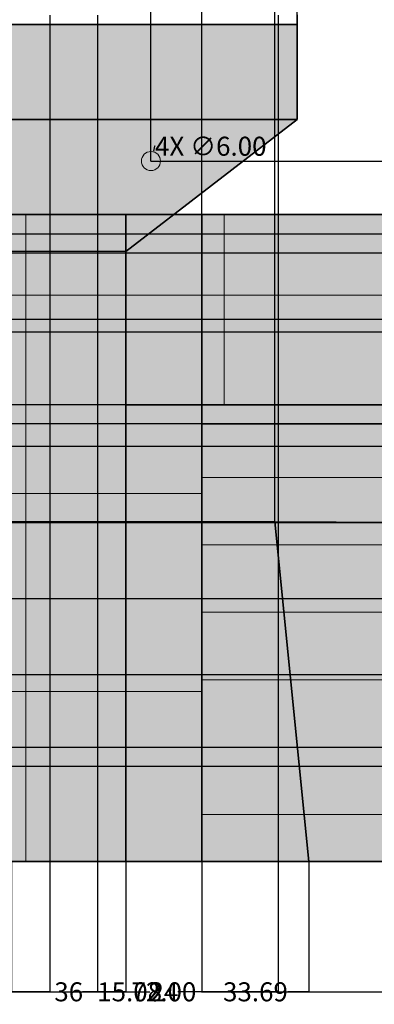
# Model space of a CAD drawing. Units: inches. Extents: x 148 to 1080, y 89 to 707.
# Tile 8 of 12: x 686 to 797, y 89 to 399. Entities that reach past the tile are written whole.
import ezdxf

# ---------------------------------------------------------------- set-up
doc = ezdxf.new("R2010")
doc.units = ezdxf.units.IN
doc.header["$MEASUREMENT"] = 0
for name, color, linetype, lineweight in [('A-ANNO-DIMS', 2, 'Continuous', 18), ('A-ELEV', 7, 'Continuous', 35), ('A-ELEV-PATT', 8, 'Continuous', 13), ('E-LITE', 3, 'Continuous', 18)]:
    doc.layers.add(name, color=color, linetype=linetype, lineweight=lineweight)
doc.styles.get("Standard").update_dxf_attribs({"font": 'arial.ttf'})
doc.dimstyles.get("Standard").update_dxf_attribs({"dimtxt": 6, "dimasz": 0.18, "dimexe": 0.18, "dimexo": 0.0625, "dimgap": 0.09, "dimtad": 0, "dimtih": 1, "dimtoh": 1, "dimdec": 0, "dimzin": 0, "dimdsep": 46, "dimlunit": 3, "dimtxsty": 'Standard', "dimcen": 0.09, "dimadec": 0, "dimazin": 0, "dimtfac": 1, "dimtdec": 0, "dimtofl": 0, "dimtmove": 0, "dimatfit": 3, "dimfxl": 1, "dimtolj": 1, "dimtzin": 0, "dimarcsym": 0})

# ---------------------------------------------------------------- blocks, each defined once
blk = doc.blocks.new('*D1')
at = {"layer": 'A-ANNO-DIMS', "color": 0, "lineweight": -2, "transparency": 16777216}
for p, q in [((215.02, 662.01), (215.02, 703.28)), ((215.2, 703.1), (604.32, 703.1)), ((1006.77, 703.1), (617.65, 703.1)), ((1006.95, 338.01), (1006.95, 703.28))]:
    blk.add_line(p, q, dxfattribs=at)
at = {"layer": 'A-ANNO-DIMS', "color": 0, "transparency": 16777216}
for points in [[(215.2, 703.13), (215.2, 703.07), (215.02, 703.1)], [(1006.77, 703.13), (1006.77, 703.07), (1006.95, 703.1)]]:
    blk.add_solid(points, dxfattribs=at)
at = {"layer": 'Defpoints', "color": 0, "transparency": 16777216}
for p in [(1006.95, 703.1), (215.02, 661.95), (1006.95, 337.95)]:
    blk.add_point(p, dxfattribs=at)
at = {"layer": 'A-ANNO-DIMS', "color": 0, "transparency": 16777216, "insert": (610.98, 703.1), "char_height": 6, "attachment_point": 5}
blk.add_mtext('\\A1;792', dxfattribs=at)
blk = doc.blocks.new('*D4')
at = {"layer": 'A-ANNO-DIMS', "color": 0, "lineweight": -2, "transparency": 16777216}
for p, q in [((683.02, 133.88), (683.02, 92.62)), ((719.02, 133.88), (719.02, 92.62)), ((683.2, 92.8), (696.64, 92.8)), ((718.84, 92.8), (705.4, 92.8))]:
    blk.add_line(p, q, dxfattribs=at)
at = {"layer": 'A-ANNO-DIMS', "color": 0, "transparency": 16777216}
for points in [[(683.2, 92.83), (683.2, 92.77), (683.02, 92.8)], [(718.84, 92.83), (718.84, 92.77), (719.02, 92.8)]]:
    blk.add_solid(points, dxfattribs=at)
at = {"layer": 'Defpoints', "color": 0, "transparency": 16777216}
for p in [(683.02, 133.95), (719.02, 133.95), (719.02, 92.8)]:
    blk.add_point(p, dxfattribs=at)
at = {"layer": 'A-ANNO-DIMS', "color": 0, "transparency": 16777216, "insert": (701.02, 92.8), "char_height": 6, "attachment_point": 5}
blk.add_mtext('\\A1;36', dxfattribs=at)
blk = doc.blocks.new('*D5')
at = {"layer": 'A-ANNO-DIMS', "color": 0, "lineweight": -2, "transparency": 16777216}
for p, q in [((719.02, 133.88), (719.02, 92.62)), ((743.02, 133.88), (743.02, 92.62)), ((719.2, 92.8), (726.59, 92.8)), ((742.84, 92.8), (735.45, 92.8))]:
    blk.add_line(p, q, dxfattribs=at)
at = {"layer": 'A-ANNO-DIMS', "color": 0, "transparency": 16777216}
for points in [[(719.2, 92.83), (719.2, 92.77), (719.02, 92.8)], [(742.84, 92.83), (742.84, 92.77), (743.02, 92.8)]]:
    blk.add_solid(points, dxfattribs=at)
at = {"layer": 'Defpoints', "color": 0, "transparency": 16777216}
for p in [(719.02, 133.95), (743.02, 133.95), (743.02, 92.8)]:
    blk.add_point(p, dxfattribs=at)
at = {"layer": 'A-ANNO-DIMS', "color": 0, "transparency": 16777216, "insert": (731.02, 92.8), "char_height": 6, "attachment_point": 5}
blk.add_mtext('\\A1;24', dxfattribs=at)
blk = doc.blocks.new('*D6')
at = {"layer": 'A-ANNO-DIMS', "color": 0, "lineweight": -2, "transparency": 16777216}
for p, q in [((743.02, 133.88), (743.02, 92.62)), ((946.95, 133.88), (946.95, 92.62)), ((743.2, 92.8), (832.39, 92.8)), ((946.77, 92.8), (857.58, 92.8))]:
    blk.add_line(p, q, dxfattribs=at)
at = {"layer": 'A-ANNO-DIMS', "color": 0, "transparency": 16777216}
for points in [[(743.2, 92.83), (743.2, 92.77), (743.02, 92.8)], [(946.77, 92.83), (946.77, 92.77), (946.95, 92.8)]]:
    blk.add_solid(points, dxfattribs=at)
at = {"layer": 'Defpoints', "color": 0, "transparency": 16777216}
for p in [(743.02, 133.95), (946.95, 133.95), (946.95, 92.8)]:
    blk.add_point(p, dxfattribs=at)
at = {"layer": 'A-ANNO-DIMS', "color": 0, "transparency": 16777216, "insert": (844.98, 92.8), "char_height": 6, "attachment_point": 5}
blk.add_mtext('\\A1;203.93', dxfattribs=at)
blk = doc.blocks.new('*D17')
at = {"layer": 'A-ANNO-DIMS', "color": 0, "lineweight": -2, "transparency": 16777216}
for p, q in [((743.02, 338.01), (743.02, 703.28)), ((743.2, 703.1), (753.64, 703.1)), ((772.84, 703.1), (762.39, 703.1)), ((773.02, 368.01), (773.02, 703.28))]:
    blk.add_line(p, q, dxfattribs=at)
at = {"layer": 'A-ANNO-DIMS', "color": 0, "transparency": 16777216}
for points in [[(743.2, 703.13), (743.2, 703.07), (743.02, 703.1)], [(772.84, 703.13), (772.84, 703.07), (773.02, 703.1)]]:
    blk.add_solid(points, dxfattribs=at)
at = {"layer": 'Defpoints', "color": 0, "transparency": 16777216}
for p in [(773.02, 703.1), (773.02, 367.95), (743.02, 337.95)]:
    blk.add_point(p, dxfattribs=at)
at = {"layer": 'A-ANNO-DIMS', "color": 0, "transparency": 16777216, "insert": (758.02, 703.1), "char_height": 6, "attachment_point": 5}
blk.add_mtext('\\A1;30', dxfattribs=at)
blk = doc.blocks.new('*D18')
at = {"layer": 'A-ANNO-DIMS', "color": 0, "lineweight": -2, "transparency": 16777216}
for p, q in [((635.08, 661.95), (1064.5, 661.95)), ((1064.32, 661.77), (1064.32, 401.1)), ((1064.32, 134.13), (1064.32, 394.79)), ((1007.01, 133.95), (1064.5, 133.95))]:
    blk.add_line(p, q, dxfattribs=at)
at = {"layer": 'A-ANNO-DIMS', "color": 0, "transparency": 16777216}
for points in [[(1064.29, 661.77), (1064.35, 661.77), (1064.32, 661.95)], [(1064.29, 134.13), (1064.35, 134.13), (1064.32, 133.95)]]:
    blk.add_solid(points, dxfattribs=at)
at = {"layer": 'Defpoints', "color": 0, "transparency": 16777216}
for p in [(635.02, 661.95), (1064.32, 661.95), (1006.95, 133.95)]:
    blk.add_point(p, dxfattribs=at)
at = {"layer": 'A-ANNO-DIMS', "color": 0, "transparency": 16777216, "insert": (1064.32, 397.95), "char_height": 6, "attachment_point": 5}
blk.add_mtext('\\A1;528', dxfattribs=at)
blk = doc.blocks.new('*D35')
at = {"layer": 'A-ANNO-DIMS', "color": 0, "lineweight": -2, "transparency": 16777216}
for p, q in [((743.02, 272.01), (743.02, 703.28)), ((743.2, 703.1), (765.77, 703.1)), ((765.95, 241.16), (765.95, 703.28)), ((765.95, 703.1), (766.13, 703.1))]:
    blk.add_line(p, q, dxfattribs=at)
at = {"layer": 'A-ANNO-DIMS', "color": 0, "transparency": 16777216}
for points in [[(743.2, 703.13), (743.2, 703.07), (743.02, 703.1)], [(765.77, 703.13), (765.77, 703.07), (765.95, 703.1)]]:
    blk.add_solid(points, dxfattribs=at)
at = {"layer": 'Defpoints', "color": 0, "transparency": 16777216}
for p in [(765.95, 703.1), (743.02, 271.95), (765.95, 241.1)]:
    blk.add_point(p, dxfattribs=at)
at = {"layer": 'A-ANNO-DIMS', "color": 0, "transparency": 16777216, "insert": (778.73, 703.1), "char_height": 6, "attachment_point": 5}
blk.add_mtext('\\A1;22.928', dxfattribs=at)
blk = doc.blocks.new('*D36')
at = {"layer": 'A-ANNO-DIMS', "color": 0, "lineweight": -2, "transparency": 16777216}
for p, q in [((765.95, 241.16), (765.95, 703.28)), ((766.13, 703.1), (844.01, 703.1)), ((934.77, 703.1), (856.89, 703.1)), ((934.95, 272.01), (934.95, 703.28))]:
    blk.add_line(p, q, dxfattribs=at)
at = {"layer": 'A-ANNO-DIMS', "color": 0, "transparency": 16777216}
for points in [[(766.13, 703.13), (766.13, 703.07), (765.95, 703.1)], [(934.77, 703.13), (934.77, 703.07), (934.95, 703.1)]]:
    blk.add_solid(points, dxfattribs=at)
at = {"layer": 'Defpoints', "color": 0, "transparency": 16777216}
for p in [(934.95, 703.1), (934.95, 271.95), (765.95, 241.1)]:
    blk.add_point(p, dxfattribs=at)
at = {"layer": 'A-ANNO-DIMS', "color": 0, "transparency": 16777216, "insert": (850.45, 703.1), "char_height": 6, "attachment_point": 5}
blk.add_mtext('\\A1;169', dxfattribs=at)
blk = doc.blocks.new('*D37')
at = {"layer": 'A-ANNO-DIMS', "color": 0, "lineweight": -2, "transparency": 16777216}
for p, q in [((765.95, 241.16), (765.95, 703.28)), ((766.13, 703.1), (836.75, 703.1)), ((927.28, 703.1), (856.66, 703.1)), ((927.46, 240.26), (927.46, 703.28))]:
    blk.add_line(p, q, dxfattribs=at)
at = {"layer": 'A-ANNO-DIMS', "color": 0, "transparency": 16777216}
for points in [[(766.13, 703.13), (766.13, 703.07), (765.95, 703.1)], [(927.28, 703.13), (927.28, 703.07), (927.46, 703.1)]]:
    blk.add_solid(points, dxfattribs=at)
at = {"layer": 'Defpoints', "color": 0, "transparency": 16777216}
for p in [(927.46, 703.1), (765.95, 241.1), (927.46, 240.2)]:
    blk.add_point(p, dxfattribs=at)
at = {"layer": 'A-ANNO-DIMS', "color": 0, "transparency": 16777216, "insert": (846.7, 703.1), "char_height": 6, "attachment_point": 5}
blk.add_mtext('\\A1;161.5', dxfattribs=at)
blk = doc.blocks.new('*D38')
at = {"layer": 'A-ANNO-DIMS', "color": 0, "lineweight": -2, "transparency": 16777216}
for p, q in [((934.89, 271.95), (160.42, 271.95)), ((160.6, 271.77), (160.6, 206.1)), ((160.6, 134.13), (160.6, 199.79)), ((934.89, 133.95), (160.42, 133.95))]:
    blk.add_line(p, q, dxfattribs=at)
at = {"layer": 'A-ANNO-DIMS', "color": 0, "transparency": 16777216}
for points in [[(160.57, 271.77), (160.63, 271.77), (160.6, 271.95)], [(160.57, 134.13), (160.63, 134.13), (160.6, 133.95)]]:
    blk.add_solid(points, dxfattribs=at)
at = {"layer": 'Defpoints', "color": 0, "transparency": 16777216}
for p in [(934.95, 271.95), (160.6, 133.95), (934.95, 133.95)]:
    blk.add_point(p, dxfattribs=at)
at = {"layer": 'A-ANNO-DIMS', "color": 0, "transparency": 16777216, "insert": (160.6, 202.95), "char_height": 6, "attachment_point": 5}
blk.add_mtext('\\A1;138', dxfattribs=at)
blk = doc.blocks.new('*D39')
at = {"layer": 'A-ANNO-DIMS', "color": 0, "lineweight": -2, "transparency": 16777216}
for p, q in [((946.89, 337.95), (160.42, 337.95)), ((160.6, 337.77), (160.6, 311.1)), ((160.6, 278.13), (160.6, 304.79)), ((946.89, 277.95), (160.42, 277.95))]:
    blk.add_line(p, q, dxfattribs=at)
at = {"layer": 'A-ANNO-DIMS', "color": 0, "transparency": 16777216}
for points in [[(160.57, 337.77), (160.63, 337.77), (160.6, 337.95)], [(160.57, 278.13), (160.63, 278.13), (160.6, 277.95)]]:
    blk.add_solid(points, dxfattribs=at)
at = {"layer": 'Defpoints', "color": 0, "transparency": 16777216}
for p in [(160.6, 337.95), (946.95, 337.95), (946.95, 277.95)]:
    blk.add_point(p, dxfattribs=at)
at = {"layer": 'A-ANNO-DIMS', "color": 0, "transparency": 16777216, "insert": (160.6, 307.95), "char_height": 6, "attachment_point": 5}
blk.add_mtext('\\A1;60', dxfattribs=at)
blk = doc.blocks.new('*D42')
at = {"layer": 'A-ANNO-DIMS', "color": 0, "lineweight": -2, "transparency": 16777216}
for p, q in [((772.96, 367.95), (160.42, 367.95)), ((160.6, 367.77), (160.6, 350.31)), ((160.6, 326.54), (160.6, 344)), ((718.96, 326.36), (160.42, 326.36))]:
    blk.add_line(p, q, dxfattribs=at)
at = {"layer": 'A-ANNO-DIMS', "color": 0, "transparency": 16777216}
for points in [[(160.57, 367.77), (160.63, 367.77), (160.6, 367.95)], [(160.57, 326.54), (160.63, 326.54), (160.6, 326.36)]]:
    blk.add_solid(points, dxfattribs=at)
at = {"layer": 'Defpoints', "color": 0, "transparency": 16777216}
for p in [(773.02, 367.95), (160.6, 326.36), (719.02, 326.36)]:
    blk.add_point(p, dxfattribs=at)
at = {"layer": 'A-ANNO-DIMS', "color": 0, "transparency": 16777216, "insert": (160.6, 347.16), "char_height": 6, "attachment_point": 5}
blk.add_mtext('\\A1;41.584', dxfattribs=at)
blk = doc.blocks.new('*D43')
at = {"layer": 'A-ANNO-DIMS', "color": 0, "lineweight": -2, "transparency": 16777216}
for p, q in [((765.88, 241.1), (160.42, 241.1)), ((160.6, 240.92), (160.6, 190.68)), ((160.6, 134.13), (160.6, 184.37)), ((776.65, 133.95), (160.42, 133.95))]:
    blk.add_line(p, q, dxfattribs=at)
at = {"layer": 'A-ANNO-DIMS', "color": 0, "transparency": 16777216}
for points in [[(160.57, 240.92), (160.63, 240.92), (160.6, 241.1)], [(160.57, 134.13), (160.63, 134.13), (160.6, 133.95)]]:
    blk.add_solid(points, dxfattribs=at)
at = {"layer": 'Defpoints', "color": 0, "transparency": 16777216}
for p in [(765.95, 241.1), (160.6, 133.95), (776.71, 133.95)]:
    blk.add_point(p, dxfattribs=at)
at = {"layer": 'A-ANNO-DIMS', "color": 0, "transparency": 16777216, "insert": (160.6, 187.52), "char_height": 6, "attachment_point": 5}
blk.add_mtext('\\A1;107.15', dxfattribs=at)
blk = doc.blocks.new('*D48')
at = {"layer": 'A-ANNO-DIMS', "color": 0, "lineweight": -2, "transparency": 16777216}
for p, q in [((683.02, 338.01), (683.02, 703.28)), ((683.2, 703.1), (694.68, 703.1)), ((726.76, 703.1), (715.28, 703.1)), ((726.94, 354.92), (726.94, 703.28))]:
    blk.add_line(p, q, dxfattribs=at)
at = {"layer": 'A-ANNO-DIMS', "color": 0, "transparency": 16777216}
for points in [[(683.2, 703.13), (683.2, 703.07), (683.02, 703.1)], [(726.76, 703.13), (726.76, 703.07), (726.94, 703.1)]]:
    blk.add_solid(points, dxfattribs=at)
at = {"layer": 'Defpoints', "color": 0, "transparency": 16777216}
for p in [(726.94, 703.1), (726.94, 354.86), (683.02, 337.95)]:
    blk.add_point(p, dxfattribs=at)
at = {"layer": 'A-ANNO-DIMS', "color": 0, "transparency": 16777216, "insert": (704.98, 703.1), "char_height": 6, "attachment_point": 5}
blk.add_mtext('\\A1;43.92', dxfattribs=at)
blk = doc.blocks.new('*D50')
at = {"layer": 'A-ANNO-DIMS', "color": 0, "lineweight": -2, "transparency": 16777216}
for p, q in [((727, 354.86), (1064.5, 354.86)), ((1064.32, 354.68), (1064.32, 349.56)), ((1064.32, 338.13), (1064.32, 343.25)), ((683.08, 337.95), (1064.5, 337.95))]:
    blk.add_line(p, q, dxfattribs=at)
at = {"layer": 'A-ANNO-DIMS', "color": 0, "transparency": 16777216}
for points in [[(1064.29, 354.68), (1064.35, 354.68), (1064.32, 354.86)], [(1064.29, 338.13), (1064.35, 338.13), (1064.32, 337.95)]]:
    blk.add_solid(points, dxfattribs=at)
at = {"layer": 'Defpoints', "color": 0, "transparency": 16777216}
for p in [(726.94, 354.86), (683.02, 337.95), (1064.32, 337.95)]:
    blk.add_point(p, dxfattribs=at)
at = {"layer": 'A-ANNO-DIMS', "color": 0, "transparency": 16777216, "insert": (1064.32, 346.4), "char_height": 6, "attachment_point": 5}
blk.add_mtext('\\A1;16.912', dxfattribs=at)
blk = doc.blocks.new('*D58')
at = {"layer": 'A-ANNO-DIMS', "color": 0, "lineweight": -2, "transparency": 16777216}
for p, q in [((611.02, 400.88), (611.02, 92.62)), ((695.02, 400.88), (695.02, 92.62)), ((611.2, 92.8), (642.81, 92.8)), ((694.84, 92.8), (663.23, 92.8))]:
    blk.add_line(p, q, dxfattribs=at)
at = {"layer": 'A-ANNO-DIMS', "color": 0, "transparency": 16777216}
for points in [[(611.2, 92.83), (611.2, 92.77), (611.02, 92.8)], [(694.84, 92.83), (694.84, 92.77), (695.02, 92.8)]]:
    blk.add_solid(points, dxfattribs=at)
at = {"layer": 'Defpoints', "color": 0, "transparency": 16777216}
for p in [(611.02, 400.95), (695.02, 400.95), (695.02, 92.8)]:
    blk.add_point(p, dxfattribs=at)
at = {"layer": 'A-ANNO-DIMS', "color": 0, "transparency": 16777216, "insert": (653.02, 92.8), "char_height": 6, "attachment_point": 5}
blk.add_mtext('\\A1;84.00', dxfattribs=at)
blk = doc.blocks.new('*D59')
at = {"layer": 'A-ANNO-DIMS', "color": 0, "lineweight": -2, "transparency": 16777216}
for p, q in [((695.02, 400.88), (695.02, 92.62)), ((767.02, 400.88), (767.02, 92.62)), ((695.2, 92.8), (720.84, 92.8)), ((766.84, 92.8), (741.2, 92.8))]:
    blk.add_line(p, q, dxfattribs=at)
at = {"layer": 'A-ANNO-DIMS', "color": 0, "transparency": 16777216}
for points in [[(695.2, 92.83), (695.2, 92.77), (695.02, 92.8)], [(766.84, 92.83), (766.84, 92.77), (767.02, 92.8)]]:
    blk.add_solid(points, dxfattribs=at)
at = {"layer": 'Defpoints', "color": 0, "transparency": 16777216}
for p in [(695.02, 400.95), (767.02, 400.95), (767.02, 92.8)]:
    blk.add_point(p, dxfattribs=at)
at = {"layer": 'A-ANNO-DIMS', "color": 0, "transparency": 16777216, "insert": (731.02, 92.8), "char_height": 6, "attachment_point": 5}
blk.add_mtext('\\A1;72.00', dxfattribs=at)
blk = doc.blocks.new('*D60')
at = {"layer": 'A-ANNO-DIMS', "color": 0, "lineweight": -2, "transparency": 16777216}
for p, q in [((695.02, 400.88), (695.02, 92.62)), ((710.1, 400.88), (710.1, 92.62)), ((695.2, 92.8), (709.92, 92.8)), ((710.1, 92.8), (710.28, 92.8))]:
    blk.add_line(p, q, dxfattribs=at)
at = {"layer": 'A-ANNO-DIMS', "color": 0, "transparency": 16777216}
for points in [[(695.2, 92.83), (695.2, 92.77), (695.02, 92.8)], [(709.92, 92.83), (709.92, 92.77), (710.1, 92.8)]]:
    blk.add_solid(points, dxfattribs=at)
at = {"layer": 'Defpoints', "color": 0, "transparency": 16777216}
for p in [(695.02, 400.95), (710.1, 400.95), (710.1, 92.8)]:
    blk.add_point(p, dxfattribs=at)
at = {"layer": 'A-ANNO-DIMS', "color": 0, "transparency": 16777216, "insert": (720.22, 92.8), "char_height": 6, "attachment_point": 5}
blk.add_mtext('\\A1;15.08', dxfattribs=at)
blk = doc.blocks.new('*D71')
at = {"layer": 'A-ANNO-DIMS', "color": 0, "lineweight": -2, "transparency": 16777216}
for p, q in [((389.08, 169.95), (1064.5, 169.95)), ((1064.32, 169.95), (1064.32, 170.13)), ((1064.32, 170.13), (1064.5, 170.13)), ((1064.32, 164.13), (1064.32, 169.77)), ((395.08, 163.95), (1064.5, 163.95))]:
    blk.add_line(p, q, dxfattribs=at)
at = {"layer": 'A-ANNO-DIMS', "color": 0, "transparency": 16777216}
for points in [[(1064.29, 169.77), (1064.35, 169.77), (1064.32, 169.95)], [(1064.29, 164.13), (1064.35, 164.13), (1064.32, 163.95)]]:
    blk.add_solid(points, dxfattribs=at)
at = {"layer": 'Defpoints', "color": 0, "transparency": 16777216}
for p in [(389.02, 169.95), (1064.32, 169.95), (395.02, 163.95)]:
    blk.add_point(p, dxfattribs=at)
at = {"layer": 'A-ANNO-DIMS', "color": 0, "transparency": 16777216, "insert": (1072.39, 170.13), "char_height": 6, "attachment_point": 5}
blk.add_mtext('\\A1;6.00', dxfattribs=at)
blk = doc.blocks.new('*D72')
at = {"layer": 'A-ANNO-DIMS', "color": 0, "lineweight": -2, "transparency": 16777216}
for p, q in [((389.08, 192.87), (1064.5, 192.87)), ((1064.32, 192.69), (1064.32, 184.56)), ((1064.32, 170.13), (1064.32, 178.26)), ((389.08, 169.95), (1064.5, 169.95))]:
    blk.add_line(p, q, dxfattribs=at)
at = {"layer": 'A-ANNO-DIMS', "color": 0, "transparency": 16777216}
for points in [[(1064.29, 192.69), (1064.35, 192.69), (1064.32, 192.87)], [(1064.29, 170.13), (1064.35, 170.13), (1064.32, 169.95)]]:
    blk.add_solid(points, dxfattribs=at)
at = {"layer": 'Defpoints', "color": 0, "transparency": 16777216}
for p in [(389.02, 192.87), (1064.32, 192.87), (389.02, 169.95)]:
    blk.add_point(p, dxfattribs=at)
at = {"layer": 'A-ANNO-DIMS', "color": 0, "transparency": 16777216, "insert": (1064.32, 181.41), "char_height": 6, "attachment_point": 5}
blk.add_mtext('\\A1;22.92', dxfattribs=at)
blk = doc.blocks.new('*D73')
at = {"layer": 'A-ANNO-DIMS', "color": 0, "lineweight": -2, "transparency": 16777216}
for p, q in [((389.08, 216.87), (1064.5, 216.87)), ((1064.32, 216.69), (1064.32, 208.02)), ((1064.32, 193.05), (1064.32, 201.72)), ((389.08, 192.87), (1064.5, 192.87))]:
    blk.add_line(p, q, dxfattribs=at)
at = {"layer": 'A-ANNO-DIMS', "color": 0, "transparency": 16777216}
for points in [[(1064.29, 216.69), (1064.35, 216.69), (1064.32, 216.87)], [(1064.29, 193.05), (1064.35, 193.05), (1064.32, 192.87)]]:
    blk.add_solid(points, dxfattribs=at)
at = {"layer": 'Defpoints', "color": 0, "transparency": 16777216}
for p in [(389.02, 216.87), (1064.32, 216.87), (389.02, 192.87)]:
    blk.add_point(p, dxfattribs=at)
at = {"layer": 'A-ANNO-DIMS', "color": 0, "transparency": 16777216, "insert": (1064.32, 204.87), "char_height": 6, "attachment_point": 5}
blk.add_mtext('\\A1;24.00', dxfattribs=at)
blk = doc.blocks.new('*D74')
at = {"layer": 'A-ANNO-DIMS', "color": 0, "lineweight": -2, "transparency": 16777216}
for p, q in [((389.08, 240.87), (1064.5, 240.87)), ((1064.32, 240.69), (1064.32, 232.02)), ((1064.32, 217.05), (1064.32, 225.72)), ((389.08, 216.87), (1064.5, 216.87))]:
    blk.add_line(p, q, dxfattribs=at)
at = {"layer": 'A-ANNO-DIMS', "color": 0, "transparency": 16777216}
for points in [[(1064.29, 240.69), (1064.35, 240.69), (1064.32, 240.87)], [(1064.29, 217.05), (1064.35, 217.05), (1064.32, 216.87)]]:
    blk.add_solid(points, dxfattribs=at)
at = {"layer": 'Defpoints', "color": 0, "transparency": 16777216}
for p in [(389.02, 240.87), (1064.32, 240.87), (389.02, 216.87)]:
    blk.add_point(p, dxfattribs=at)
at = {"layer": 'A-ANNO-DIMS', "color": 0, "transparency": 16777216, "insert": (1064.32, 228.87), "char_height": 6, "attachment_point": 5}
blk.add_mtext('\\A1;24.00', dxfattribs=at)
blk = doc.blocks.new('*D75')
at = {"layer": 'A-ANNO-DIMS', "color": 0, "lineweight": -2, "transparency": 16777216}
for p, q in [((389.08, 264.87), (1064.5, 264.87)), ((1064.32, 264.69), (1064.32, 256.02)), ((1064.32, 241.05), (1064.32, 249.72)), ((389.08, 240.87), (1064.5, 240.87))]:
    blk.add_line(p, q, dxfattribs=at)
at = {"layer": 'A-ANNO-DIMS', "color": 0, "transparency": 16777216}
for points in [[(1064.29, 264.69), (1064.35, 264.69), (1064.32, 264.87)], [(1064.29, 241.05), (1064.35, 241.05), (1064.32, 240.87)]]:
    blk.add_solid(points, dxfattribs=at)
at = {"layer": 'Defpoints', "color": 0, "transparency": 16777216}
for p in [(389.02, 264.87), (1064.32, 264.87), (389.02, 240.87)]:
    blk.add_point(p, dxfattribs=at)
at = {"layer": 'A-ANNO-DIMS', "color": 0, "transparency": 16777216, "insert": (1064.32, 252.87), "char_height": 6, "attachment_point": 5}
blk.add_mtext('\\A1;24.00', dxfattribs=at)
blk = doc.blocks.new('*D76')
at = {"layer": 'A-ANNO-DIMS', "color": 0, "lineweight": -2, "transparency": 16777216}
for p, q in [((389.08, 300.95), (1064.5, 300.95)), ((1064.32, 300.77), (1064.32, 286.06)), ((1064.32, 265.05), (1064.32, 279.75)), ((389.08, 264.87), (1064.5, 264.87))]:
    blk.add_line(p, q, dxfattribs=at)
at = {"layer": 'A-ANNO-DIMS', "color": 0, "transparency": 16777216}
for points in [[(1064.29, 300.77), (1064.35, 300.77), (1064.32, 300.95)], [(1064.29, 265.05), (1064.35, 265.05), (1064.32, 264.87)]]:
    blk.add_solid(points, dxfattribs=at)
at = {"layer": 'Defpoints', "color": 0, "transparency": 16777216}
for p in [(389.02, 300.95), (1064.32, 300.95), (389.02, 264.87)]:
    blk.add_point(p, dxfattribs=at)
at = {"layer": 'A-ANNO-DIMS', "color": 0, "transparency": 16777216, "insert": (1064.32, 282.91), "char_height": 6, "attachment_point": 5}
blk.add_mtext('\\A1;36.08', dxfattribs=at)
blk = doc.blocks.new('*D77')
at = {"layer": 'A-ANNO-DIMS', "color": 0, "lineweight": -2, "transparency": 16777216}
for p, q in [((389.08, 304.95), (1064.5, 304.95)), ((1064.32, 304.95), (1064.32, 305.13)), ((1064.32, 305.13), (1064.5, 305.13)), ((1064.32, 301.13), (1064.32, 304.77)), ((389.08, 300.95), (1064.5, 300.95))]:
    blk.add_line(p, q, dxfattribs=at)
at = {"layer": 'A-ANNO-DIMS', "color": 0, "transparency": 16777216}
for points in [[(1064.29, 304.77), (1064.35, 304.77), (1064.32, 304.95)], [(1064.29, 301.13), (1064.35, 301.13), (1064.32, 300.95)]]:
    blk.add_solid(points, dxfattribs=at)
at = {"layer": 'Defpoints', "color": 0, "transparency": 16777216}
for p in [(389.02, 304.95), (1064.32, 304.95), (389.02, 300.95)]:
    blk.add_point(p, dxfattribs=at)
at = {"layer": 'A-ANNO-DIMS', "color": 0, "transparency": 16777216, "insert": (1072.5, 305.13), "char_height": 6, "attachment_point": 5}
blk.add_mtext('\\A1;4.00', dxfattribs=at)
blk = doc.blocks.new('*D78')
at = {"layer": 'A-ANNO-DIMS', "color": 0, "lineweight": -2, "transparency": 16777216}
for p, q in [((389.08, 325.95), (1064.5, 325.95)), ((1064.32, 325.77), (1064.32, 318.6)), ((1064.32, 305.13), (1064.32, 312.29)), ((389.08, 304.95), (1064.5, 304.95))]:
    blk.add_line(p, q, dxfattribs=at)
at = {"layer": 'A-ANNO-DIMS', "color": 0, "transparency": 16777216}
for points in [[(1064.29, 325.77), (1064.35, 325.77), (1064.32, 325.95)], [(1064.29, 305.13), (1064.35, 305.13), (1064.32, 304.95)]]:
    blk.add_solid(points, dxfattribs=at)
at = {"layer": 'Defpoints', "color": 0, "transparency": 16777216}
for p in [(389.02, 325.95), (1064.32, 325.95), (389.02, 304.95)]:
    blk.add_point(p, dxfattribs=at)
at = {"layer": 'A-ANNO-DIMS', "color": 0, "transparency": 16777216, "insert": (1064.32, 315.45), "char_height": 6, "attachment_point": 5}
blk.add_mtext('\\A1;21.00', dxfattribs=at)
blk = doc.blocks.new('*D79')
at = {"layer": 'A-ANNO-DIMS', "color": 0, "lineweight": -2, "transparency": 16777216}
for p, q in [((395.08, 331.95), (1064.5, 331.95)), ((1064.32, 331.95), (1064.32, 332.13)), ((1064.32, 332.13), (1064.5, 332.13)), ((1064.32, 326.13), (1064.32, 331.77)), ((389.08, 325.95), (1064.5, 325.95))]:
    blk.add_line(p, q, dxfattribs=at)
at = {"layer": 'A-ANNO-DIMS', "color": 0, "transparency": 16777216}
for points in [[(1064.29, 331.77), (1064.35, 331.77), (1064.32, 331.95)], [(1064.29, 326.13), (1064.35, 326.13), (1064.32, 325.95)]]:
    blk.add_solid(points, dxfattribs=at)
at = {"layer": 'Defpoints', "color": 0, "transparency": 16777216}
for p in [(395.02, 331.95), (1064.32, 331.95), (389.02, 325.95)]:
    blk.add_point(p, dxfattribs=at)
at = {"layer": 'A-ANNO-DIMS', "color": 0, "transparency": 16777216, "insert": (1072.39, 332.13), "char_height": 6, "attachment_point": 5}
blk.add_mtext('\\A1;6.00', dxfattribs=at)
blk = doc.blocks.new('*D100')
at = {"layer": 'A-ANNO-DIMS', "color": 0, "lineweight": -2, "transparency": 16777216}
for p, q in [((743.02, 133.88), (743.02, 92.62)), ((776.71, 133.88), (776.71, 92.62)), ((743.2, 92.8), (749.65, 92.8)), ((776.53, 92.8), (770.08, 92.8))]:
    blk.add_line(p, q, dxfattribs=at)
at = {"layer": 'A-ANNO-DIMS', "color": 0, "transparency": 16777216}
for points in [[(743.2, 92.83), (743.2, 92.77), (743.02, 92.8)], [(776.53, 92.83), (776.53, 92.77), (776.71, 92.8)]]:
    blk.add_solid(points, dxfattribs=at)
at = {"layer": 'Defpoints', "color": 0, "transparency": 16777216}
for p in [(743.02, 133.95), (776.71, 133.95), (776.71, 92.8)]:
    blk.add_point(p, dxfattribs=at)
at = {"layer": 'A-ANNO-DIMS', "color": 0, "transparency": 16777216, "insert": (759.87, 92.8), "char_height": 6, "attachment_point": 5}
blk.add_mtext('\\A1;33.69', dxfattribs=at)
blk = doc.blocks.new('*D102')
at = {"layer": 'A-ANNO-DIMS', "color": 0, "lineweight": -2, "transparency": 16777216}
for p, q in [((742.96, 271.95), (160.42, 271.95)), ((160.6, 271.77), (160.6, 259.68)), ((160.6, 241.28), (160.6, 253.37)), ((765.88, 241.1), (160.42, 241.1))]:
    blk.add_line(p, q, dxfattribs=at)
at = {"layer": 'A-ANNO-DIMS', "color": 0, "transparency": 16777216}
for points in [[(160.57, 271.77), (160.63, 271.77), (160.6, 271.95)], [(160.57, 241.28), (160.63, 241.28), (160.6, 241.1)]]:
    blk.add_solid(points, dxfattribs=at)
at = {"layer": 'Defpoints', "color": 0, "transparency": 16777216}
for p in [(160.6, 271.95), (743.02, 271.95), (765.95, 241.1)]:
    blk.add_point(p, dxfattribs=at)
at = {"layer": 'A-ANNO-DIMS', "color": 0, "transparency": 16777216, "insert": (160.6, 256.52), "char_height": 6, "attachment_point": 5}
blk.add_mtext('\\A1;30.85', dxfattribs=at)
blk = doc.blocks.new('*D103')
at = {"layer": 'A-ANNO-DIMS', "color": 0, "lineweight": -2, "transparency": 16777216}
for p, q in [((728.07, 359.53), (727.69, 357.95)), ((728.25, 359.53), (728.07, 359.53)), ((726.85, 354.86), (727.03, 354.86)), ((726.94, 354.77), (726.94, 354.95))]:
    blk.add_line(p, q, dxfattribs=at)
at = {"layer": 'A-ANNO-DIMS', "color": 0, "transparency": 16777216}
blk.add_solid([(727.66, 357.96), (727.72, 357.94), (727.65, 357.78)], dxfattribs=at)
at = {"layer": 'Defpoints', "color": 0, "transparency": 16777216}
for p in [(727.65, 357.78), (726.24, 351.94)]:
    blk.add_point(p, dxfattribs=at)
at = {"layer": 'A-ANNO-DIMS', "color": 0, "transparency": 16777216, "insert": (745.79, 359.53), "char_height": 6, "attachment_point": 5}
blk.add_mtext('\\A1;4X ∅6.00', dxfattribs=at)

msp = doc.modelspace()

# ---------------------------------------------------------------- hatches: boundary and pattern name
at = {"layer": 'A-ELEV-PATT'}
h = msp.add_hatch(color=256, dxfattribs=at)
h.dxf.hatch_style = 1
h.paths.add_polyline_path([(635.0199, 661.9474), (611.0199, 661.9474), (215.0199, 661.9474), (215.0199, 631.9474), (611.0199, 631.9474), (635.0199, 631.9474)])
h.paths.add_polyline_path([(773.0199, 397.9474), (215.0199, 397.9474), (215.0199, 367.9474), (773.0199, 367.9474)])
h = msp.add_hatch(color=256, dxfattribs=at)
h.dxf.hatch_style = 1
h.paths.add_polyline_path([(622.6005, 631.9474), (611.0199, 631.9474), (215.0199, 631.9474), (251.0199, 542.9352), (251.0199, 601.9474), (527.0199, 601.9474), (527.0199, 541.9474), (598.6005, 541.9474)])
h.paths.add_polyline_path([(558.5775, 608.9493, -1), (552.5775, 608.9493, -1)], flags=16)
h.paths.add_polyline_path([(586.7589, 556.0652, -1), (580.7589, 556.0652, -1)], flags=16)
h.paths.add_polyline_path([(635.0199, 631.9474), (622.6005, 631.9474), (598.6005, 541.9474), (611.0199, 541.9474)])
h.paths.add_polyline_path([(773.0199, 367.9474), (215.0199, 367.9474), (251.0199, 337.9474), (251.0199, 349.9474), (527.0199, 349.9474), (527.0199, 337.9474), (734.0628, 337.9474)])
h.paths.add_polyline_path([(631.1736, 353.1958, -1), (625.1736, 353.1958, -1)], flags=16)
h.paths.add_polyline_path([(729.9419, 354.8591, -1), (723.9419, 354.8591, -1)], flags=16)
h = msp.add_hatch(color=256, dxfattribs=at)
h.dxf.hatch_style = 1
h.paths.add_polyline_path([(552.5775, 608.9493, 1), (558.5775, 608.9493, 1)])
h.paths.add_polyline_path([(586.7589, 556.0652, 1), (580.7589, 556.0652, 1)])
h.paths.add_polyline_path([(625.1736, 353.1958, 1), (631.1736, 353.1958, 1)])
h.paths.add_polyline_path([(723.9419, 354.8591, 1), (729.9419, 354.8591, 1)])
h = msp.add_hatch(color=256, dxfattribs=at)
h.dxf.hatch_style = 1
h.paths.add_polyline_path([(527.0199, 349.9474), (395.0199, 349.9474), (395.0199, 271.2774), (527.0199, 272.3839)])
h.paths.add_polyline_path([(275.0199, 349.9474), (251.0199, 349.9474), (251.0199, 270.0704), (275.0199, 270.2716)])
h.paths.add_polyline_path([(743.0199, 337.9474), (734.0628, 337.9474), (719.0199, 326.3632), (719.0199, 277.9474), (743.0199, 277.9474)])
h.paths.add_polyline_path([(743.0199, 277.9474), (719.0199, 277.9474), (719.0199, 133.9474), (743.0199, 133.9474)])
h.paths.add_polyline_path([(734.0628, 337.9474), (719.0199, 337.9474), (719.0199, 326.3632)])
h = msp.add_hatch(color=256, dxfattribs=at)
h.dxf.hatch_style = 1
h.paths.add_polyline_path([(527.0199, 272.3839), (395.0199, 271.2774), (395.0199, 163.9474), (275.0199, 163.9474), (275.0199, 270.2716), (251.0199, 270.0704), (251.0199, 133.9474), (527.0199, 133.9474)])
h.paths.add_polyline_path([(1006.9492, 337.9474), (946.9492, 337.9474), (946.9492, 277.9474), (1006.9492, 277.9474)])
h.paths.add_polyline_path([(1006.9492, 277.9474), (946.9492, 277.9474), (946.9492, 133.9474), (1006.9492, 133.9474)])
h.paths.add_polyline_path([(946.9492, 337.9474), (743.0199, 337.9474), (743.0199, 277.9474), (946.9492, 277.9474)])
h = msp.add_hatch(dxfattribs=at)
h.set_pattern_fill('ANSI37', color=256, scale=500, angle=135)
h.paths.add_polyline_path([(946.9492, 337.9474), (743.0199, 337.9474), (743.0199, 277.9474), (946.9492, 277.9474)])
h.paths.add_polyline_path([(1006.9492, 337.9474), (946.9492, 337.9474), (946.9492, 277.9474), (1006.9492, 277.9474)])
h.paths.add_polyline_path([(1006.9492, 277.9474), (946.9492, 277.9474), (946.9492, 133.9474), (1006.9492, 133.9474)])
h.paths.add_polyline_path([(719.0199, 337.9474), (683.0199, 337.9474), (683.0199, 133.9474), (719.0199, 133.9474)])
h.paths.add_polyline_path([(743.0199, 277.9474), (719.0199, 277.9474), (719.0199, 133.9474), (743.0199, 133.9474)])
h.paths.add_polyline_path([(743.0199, 337.9474), (734.0628, 337.9474), (719.0199, 326.3632), (719.0199, 277.9474), (743.0199, 277.9474)])
h.paths.add_polyline_path([(683.0199, 283.9474), (671.0199, 283.9474), (671.0199, 133.9474), (683.0199, 133.9474)])
h = msp.add_hatch(color=256, dxfattribs=at)
h.dxf.hatch_style = 1
h.paths.add_polyline_path([(719.0199, 337.9474), (683.0199, 337.9474), (683.0199, 133.9474), (719.0199, 133.9474)])
h = msp.add_hatch(color=256, dxfattribs=at)
h.dxf.hatch_style = 1
h.paths.add_polyline_path([(946.9492, 277.9474), (743.0199, 277.9474), (743.0199, 271.9474), (934.9492, 271.9474)])
h.paths.add_polyline_path([(946.9492, 277.9474), (934.9492, 271.9474), (934.9492, 133.9474), (946.9492, 133.9474)])
h = msp.add_hatch(color=256, dxfattribs=at)
h.dxf.hatch_style = 1
h.paths.add_polyline_path([(934.9492, 271.9474), (743.0199, 271.9474), (743.0199, 133.9474), (776.713, 133.9474), (765.9474, 241.0996), (922.2028, 240.1776), (927.4587, 240.1966), (927.4587, 133.9474), (934.9492, 133.9474)])
h = msp.add_hatch(dxfattribs=at)
h.set_pattern_fill('ANSI31', color=256, scale=170, angle=135)
h.paths.add_polyline_path([(927.4587, 240.1966), (922.2028, 240.1776), (765.9474, 241.0996), (776.713, 133.9474), (927.4587, 133.9474)], flags=17)
h.paths.add_polyline_path([(934.9492, 271.9474), (743.0199, 271.9474), (743.0199, 133.9474), (776.713, 133.9474), (765.9474, 241.0996), (922.2028, 240.1776), (927.4587, 240.1966), (927.4587, 133.9474), (934.9492, 133.9474)])
h = msp.add_hatch(color=256, dxfattribs=at)
h.dxf.hatch_style = 1
h.paths.add_polyline_path([(927.4587, 240.1966), (922.2028, 240.1776), (765.9474, 241.0996), (776.713, 133.9474), (927.4587, 133.9474)])

# ---------------------------------------------------------------- linework, layer by layer
at = {"layer": 'A-ELEV'}
for p, q in [((773.0199, 367.9474), (773.0199, 400.9474)), ((215.0199, 397.9474), (773.0199, 397.9474)), ((215.0199, 367.9474), (773.0199, 367.9474)), ((773.0199, 367.9474), (719.0199, 326.3632)), ((527.0199, 337.9474), (1006.9492, 337.9474)), ((719.0199, 133.9474), (719.0199, 337.9474)), ((743.0199, 133.9474), (743.0199, 337.9474)), ((719.0199, 277.9474), (1006.9492, 277.9474)), ((743.0199, 271.9474), (934.9492, 271.9474)), ((776.713, 133.9474), (765.9474, 241.0996)), ((765.9474, 241.0996), (922.2028, 240.1776)), ((201.7492, 133.9474), (1023.175, 133.9474))]:
    msp.add_line(p, q, dxfattribs=at)
at = {"layer": 'E-LITE'}
msp.add_circle((726.9419, 354.8591), 3, dxfattribs=at)

# ---------------------------------------------------------------- dimensions: what is measured, and where the dimension line sits
at = {"layer": 'A-ANNO-DIMS'}
for base, p1, p2, override, picture, middle in [((1006.9492, 703.0974), (215.0199, 661.9474), (1006.9492, 337.9474), {"dimdec": 0, "dimlfac": 1, "dimrnd": 0, "dimzin": 0, "dimdsep": 46, "dimlunit": 2}, '*D1', (610.9845, 703.0974)), ((726.9419, 703.0974), (683.0199, 337.9474), (726.9419, 354.8591), {"dimdec": 2, "dimlfac": 1, "dimrnd": 0, "dimzin": 0, "dimdsep": 46, "dimlunit": 2}, '*D48', (704.9809, 703.0974)), ((773.0199, 703.0974), (743.0199, 337.9474), (773.0199, 367.9474), {"dimdec": 0, "dimlfac": 1, "dimrnd": 0, "dimzin": 0, "dimdsep": 46, "dimlunit": 2}, '*D17', (758.0199, 703.0974)), ((765.947371, 703.097395), (743.019868, 271.947395), (765.947371, 241.09963), {"dimdec": 3, "dimlfac": 1, "dimrnd": 0, "dimzin": 0, "dimdsep": 46, "dimlunit": 2}, '*D35', (778.728967, 703.097395)), ((934.9492, 703.0974), (765.9474, 241.0996), (934.9492, 271.9474), {"dimdec": 0, "dimlfac": 1, "dimrnd": 0, "dimzin": 0, "dimdsep": 46, "dimlunit": 2}, '*D36', (850.4483, 703.0974)), ((927.4587, 703.0974), (765.9474, 241.0996), (927.4587, 240.1966), {"dimdec": 1, "dimlfac": 1, "dimrnd": 0, "dimzin": 0, "dimdsep": 46, "dimlunit": 2}, '*D37', (846.703, 703.0974)), ((695.0199, 92.7974), (611.0199, 400.9474), (695.0199, 400.9474), {"dimdec": 2, "dimlfac": 1, "dimrnd": 0, "dimzin": 0, "dimdsep": 46, "dimlunit": 2}, '*D58', (653.0199, 92.7974)), ((767.0199, 92.7974), (695.0199, 400.9474), (767.0199, 400.9474), {"dimdec": 2, "dimlfac": 1, "dimrnd": 0, "dimzin": 0, "dimdsep": 46, "dimlunit": 2}, '*D59', (731.0199, 92.7974)), ((710.0996, 92.7974), (695.0199, 400.9474), (710.0996, 400.9474), {"dimdec": 2, "dimlfac": 1, "dimrnd": 0, "dimzin": 0, "dimdsep": 46, "dimlunit": 2}, '*D60', (720.2168, 92.7974)), ((719.0199, 92.7974), (683.0199, 133.9474), (719.0199, 133.9474), {"dimdec": 0, "dimlfac": 1, "dimrnd": 0, "dimzin": 0, "dimdsep": 46, "dimlunit": 2}, '*D4', (701.0199, 92.7974)), ((743.0199, 92.7974), (719.0199, 133.9474), (743.0199, 133.9474), {"dimdec": 0, "dimlfac": 1, "dimrnd": 0, "dimzin": 0, "dimdsep": 46, "dimlunit": 2}, '*D5', (731.0199, 92.7974)), ((946.9492, 92.7974), (743.0199, 133.9474), (946.9492, 133.9474), {"dimdec": 2, "dimlfac": 1, "dimrnd": 0, "dimzin": 0, "dimdsep": 46, "dimlunit": 2}, '*D6', (844.9845, 92.7974)), ((776.713, 92.7974), (743.0199, 133.9474), (776.713, 133.9474), {"dimdec": 2, "dimlfac": 1, "dimrnd": 0, "dimzin": 0, "dimdsep": 46, "dimlunit": 2}, '*D100', (759.8664, 92.7974))]:
    dim = msp.add_linear_dim(base=base, p1=p1, p2=p2, dimstyle='Standard', override=override, dxfattribs=at)
    dim.commit()
    dim.dimension.update_dxf_attribs({"geometry": picture, "text_midpoint": middle})
for base, p1, p2, override, picture, middle in [((1064.325, 661.9474), (1006.9492, 133.9474), (635.0199, 661.9474), {"dimdec": 0, "dimlfac": 1, "dimrnd": 0, "dimzin": 0, "dimdsep": 46, "dimlunit": 2}, '*D18', (1064.325, 397.9474)), ((160.5992, 326.3632), (773.0199, 367.9474), (719.0199, 326.3632), {"dimdec": 3, "dimlfac": 1, "dimrnd": 0, "dimzin": 0, "dimdsep": 46, "dimlunit": 2}, '*D42', (160.5992, 347.1553)), ((1064.325, 337.9474), (726.9419, 354.8591), (683.0199, 337.9474), {"dimdec": 3, "dimlfac": 1, "dimrnd": 0, "dimzin": 0, "dimdsep": 46, "dimlunit": 2}, '*D50', (1064.325, 346.4032)), ((160.5992, 337.9474), (946.9492, 277.9474), (946.9492, 337.9474), {"dimdec": 0, "dimlfac": 1, "dimrnd": 0, "dimzin": 0, "dimdsep": 46, "dimlunit": 2}, '*D39', (160.5992, 307.9474)), ((1064.325, 331.9474), (389.0199, 325.9474), (395.0199, 331.9474), {"dimdec": 2, "dimlfac": 1, "dimrnd": 0, "dimzin": 0, "dimdsep": 46, "dimlunit": 2}, '*D79', (1072.3937, 332.1274)), ((1064.325, 325.9474), (389.0199, 304.9474), (389.0199, 325.9474), {"dimdec": 2, "dimlfac": 1, "dimrnd": 0, "dimzin": 0, "dimdsep": 46, "dimlunit": 2}, '*D78', (1064.325, 315.4474)), ((1064.325, 304.9474), (389.0199, 300.9474), (389.0199, 304.9474), {"dimdec": 2, "dimlfac": 1, "dimrnd": 0, "dimzin": 0, "dimdsep": 46, "dimlunit": 2}, '*D77', (1072.4981, 305.1274)), ((1064.325, 300.9474), (389.0199, 264.8696), (389.0199, 300.9474), {"dimdec": 2, "dimlfac": 1, "dimrnd": 0, "dimzin": 0, "dimdsep": 46, "dimlunit": 2}, '*D76', (1064.325, 282.9085)), ((160.5992, 271.9474), (765.9474, 241.0996), (743.0199, 271.9474), {"dimdec": 2, "dimlfac": 1, "dimrnd": 0, "dimzin": 0, "dimdsep": 46, "dimlunit": 2}, '*D102', (160.5992, 256.5235)), ((160.5992, 133.9474), (934.9492, 271.9474), (934.9492, 133.9474), {"dimdec": 0, "dimlfac": 1, "dimrnd": 0, "dimzin": 0, "dimdsep": 46, "dimlunit": 2}, '*D38', (160.5992, 202.9474)), ((1064.325, 264.8696), (389.0199, 240.8696), (389.0199, 264.8696), {"dimdec": 2, "dimlfac": 1, "dimrnd": 0, "dimzin": 0, "dimdsep": 46, "dimlunit": 2}, '*D75', (1064.325, 252.8696)), ((160.5992, 133.9474), (765.9474, 241.0996), (776.713, 133.9474), {"dimdec": 2, "dimlfac": 1, "dimrnd": 0, "dimzin": 0, "dimdsep": 46, "dimlunit": 2}, '*D43', (160.5992, 187.5235)), ((1064.325, 240.8696), (389.0199, 216.8696), (389.0199, 240.8696), {"dimdec": 2, "dimlfac": 1, "dimrnd": 0, "dimzin": 0, "dimdsep": 46, "dimlunit": 2}, '*D74', (1064.325, 228.8696)), ((1064.325, 216.8696), (389.0199, 192.8696), (389.0199, 216.8696), {"dimdec": 2, "dimlfac": 1, "dimrnd": 0, "dimzin": 0, "dimdsep": 46, "dimlunit": 2}, '*D73', (1064.325, 204.8696)), ((1064.325, 192.8696), (389.0199, 169.9474), (389.0199, 192.8696), {"dimdec": 2, "dimlfac": 1, "dimrnd": 0, "dimzin": 0, "dimdsep": 46, "dimlunit": 2}, '*D72', (1064.325, 181.4085)), ((1064.325, 169.9474), (395.0199, 163.9474), (389.0199, 169.9474), {"dimdec": 2, "dimlfac": 1, "dimrnd": 0, "dimzin": 0, "dimdsep": 46, "dimlunit": 2}, '*D71', (1072.3937, 170.1274))]:
    dim = msp.add_linear_dim(base=base, p1=p1, p2=p2, angle=90, dimstyle='Standard', override=override, dxfattribs=at)
    dim.commit()
    dim.dimension.update_dxf_attribs({"geometry": picture, "text_midpoint": middle})
dim = msp.add_diameter_dim_2p(p1=(726.2385, 351.9427), p2=(727.6453, 357.7755), text='4X <>', dimstyle='Standard', override={"dimdec": 2, "dimlfac": 1, "dimrnd": 0, "dimzin": 0, "dimdsep": 46, "dimlunit": 2}, dxfattribs=at)
dim.commit()
dim.dimension.update_dxf_attribs({"geometry": '*D103', "text_midpoint": (745.7909, 359.5253), "dimtype": 163})

doc.saveas('drawing.dxf')
